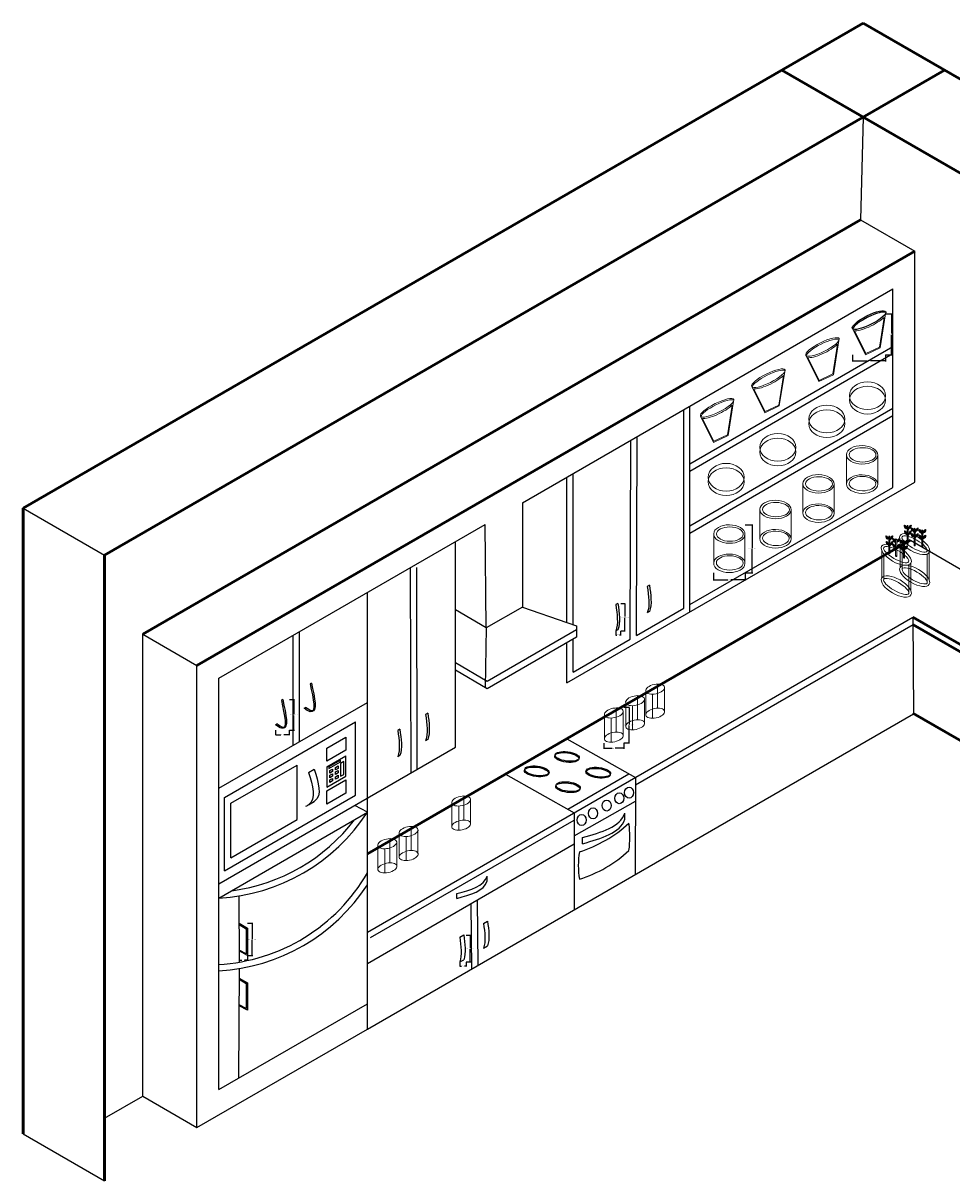
# Model space of a CAD drawing. Units: centimetres. Extents: x 16 to 604, y -284 to 166.
# Tile 1 of 2: x 16 to 312, y -204 to 166. Entities that reach past the tile are written whole.
import ezdxf

# ---------------------------------------------------------------- set-up
doc = ezdxf.new("R2010")
doc.units = ezdxf.units.CM
doc.header["$MEASUREMENT"] = 0
for name, color, linetype, lineweight in [('A-ANNO-DIMS', 2, 'Continuous', 18), ('A-EQPM', 4, 'Continuous', 25), ('A-FLOR-FIXT', 3, 'Continuous', 25), ('A-FURN-ACCS', 9, 'Continuous', 18), ('A-FURN-CASE', 8, 'Continuous', 25), ('A-WALL', 7, 'Continuous', 50)]:
    doc.layers.add(name, color=color, linetype=linetype, lineweight=lineweight)
doc.styles.get("Standard").update_dxf_attribs({"font": 'arial.ttf'})
doc.dimstyles.get("Standard").update_dxf_attribs({"dimtxt": 0.18, "dimasz": 0.18, "dimexe": 0.18, "dimexo": 0.0625, "dimgap": 0.09, "dimtad": 0, "dimtih": 1, "dimtoh": 1, "dimdec": 0, "dimzin": 0, "dimdsep": 46, "dimtxsty": 'Standard', "dimcen": 0.09, "dimadec": 0, "dimazin": 0, "dimtfac": 1, "dimtdec": 0, "dimtofl": 0, "dimtmove": 0, "dimatfit": 3, "dimfxl": 1, "dimtolj": 1, "dimtzin": 0, "dimarcsym": 0})

# ---------------------------------------------------------------- blocks, each defined once
blk = doc.blocks.new('GLASS-TUMBLER')
for p, q in [((0.02, 1.05), (0.02, 8.7)), ((2.21, 0.13), (2.21, 7.72)), ((3.82, 3.25), (3.82, 10.96)), ((6.02, 2.33), (6.02, 9.98))]:
    blk.add_line(p, q)
for centre in [(3.02, 9.34), (3.03, 1.62)]:
    blk.add_ellipse(centre, major_axis=(-3, -0.64), ratio=0.495695)
blk = doc.blocks.new('JAR-STORAGE')
for p, q in [((0, 12.4), (0, 3.03)), ((10, 12.25), (10, 2.89))]:
    blk.add_line(p, q)
for centre, major_axis, ratio in [((5, 12.32), (-5, 0.07), 0.591821), ((5.17, 12.3), (-4.28, 0.05), 0.535916), ((5, 2.96), (-5, 0.07), 0.591821), ((5.13, 3.1), (-4.28, 0.05), 0.535916)]:
    blk.add_ellipse(centre, major_axis=major_axis, ratio=ratio)
blk = doc.blocks.new('CUP')
for p, q in [((8.64, 2.46), (10.15, 11.93)), ((8.83, 2.21), (10.57, 13.1)), ((4.2, 0), (0, 8.4)), ((4.29, 0.38), (0.64, 7.69)), ((4.2, 0), (8.83, 2.21)), ((4.29, 0.38), (8.64, 2.46))]:
    blk.add_line(p, q)
blk.add_ellipse((5.52, 10.63), major_axis=(5.33, 2.67), ratio=0.250569, start_param=3.449003, end_param=5.626799)
blk = doc.blocks.new('HANDLE-FRIDGE')
for p, q in [((0, 10.27), (2.69, 8.71)), ((0, 9.85), (2.26, 8.55)), ((2.26, 8.55), (2.26, 0.52)), ((2.69, 8.71), (2.69, 0)), ((2.69, 8.3), (2.69, 8.3)), ((2.26, 0.52), (0.04, 1.71)), ((2.69, 0), (0.04, 1.42))]:
    blk.add_line(p, q)
blk = doc.blocks.new('MICROWAVE-BUTTON')
for p, q in [((0, 0.81), (0.84, 1.29)), ((0, 0), (0, 0.81)), ((0.84, 0.49), (0, 0)), ((0.84, 1.29), (0.84, 0.49))]:
    blk.add_line(p, q)
blk = doc.blocks.new('HANDLE-CAB-A')
for p, q in [((0.67, 8.79), (0, 8.4)), ((0.67, 0.39), (0, 0))]:
    blk.add_line(p, q)
for points in [[(0, 8.4), (0.44, 5.35), (0.89, 2.29), (0, 0)], [(0.67, 8.79), (1.12, 5.74), (1.56, 2.68), (0.67, 0.39)]]:
    blk.add_open_spline(points, degree=3)
blk = doc.blocks.new('HANDLE-CAB-B')
for p, q in [((2.34, 9.21), (1.89, 8.95)), ((0, 1.14), (0.45, 1.41))]:
    blk.add_line(p, q)
for points in [[(1.89, 8.95), (2.92, 4.2), (4.21, -1.72), (0.69, 0.67), (0, 1.14)], [(2.34, 9.21), (3.37, 4.46), (4.66, -1.46), (1.15, 0.93), (0.45, 1.41)]]:
    blk.add_open_spline(points, degree=3, knots=[0, 0, 0, 0, 8.893101, 11.076836, 11.076836, 11.076836, 11.076836])
blk = doc.blocks.new('HANDLE-CAB-C')
for p, q in [((0, 7.89), (1.27, 8.62)), ((0, 0), (1.27, 0.73))]:
    blk.add_line(p, q)
for points in [[(0, 7.89), (0.38, 5.04), (0.76, 2.19), (0, 0)], [(1.27, 8.62), (1.65, 5.77), (2.03, 2.92), (1.27, 0.73)]]:
    blk.add_open_spline(points, degree=3)
blk = doc.blocks.new('*D13')
at = {"layer": 'A-ANNO-DIMS', "color": 0, "lineweight": -2, "transparency": 16777216}
for p, q in [((246.35, 6.13), (248.77, 6.13)), ((248.59, 5.95), (248.59, -1.37)), ((248.59, -9.05), (248.59, -1.73)), ((246.35, -9.23), (248.77, -9.23))]:
    blk.add_line(p, q, dxfattribs=at)
at = {"layer": 'A-ANNO-DIMS', "color": 0, "transparency": 16777216}
for points in [[(248.56, 5.95), (248.62, 5.95), (248.59, 6.13)], [(248.56, -9.05), (248.62, -9.05), (248.59, -9.23)]]:
    blk.add_solid(points, dxfattribs=at)
at = {"layer": 'Defpoints', "color": 0, "transparency": 16777216}
for p in [(246.29, 6.13), (248.59, 6.13), (246.29, -9.23)]:
    blk.add_point(p, dxfattribs=at)
at = {"layer": 'A-ANNO-DIMS', "color": 0, "transparency": 16777216, "insert": (248.59, -1.55), "char_height": 0.18, "attachment_point": 5}
blk.add_mtext('\\A1;STORAGE JAR 15 TYP.', dxfattribs=at)
blk = doc.blocks.new('*D14')
at = {"layer": 'A-ANNO-DIMS', "color": 0, "lineweight": -2, "transparency": 16777216}
for p, q in [((236.24, -9.3), (236.24, -11.72)), ((246.29, -9.3), (246.29, -11.72)), ((236.42, -11.54), (240.75, -11.54)), ((246.11, -11.54), (241.78, -11.54))]:
    blk.add_line(p, q, dxfattribs=at)
at = {"layer": 'A-ANNO-DIMS', "color": 0, "transparency": 16777216}
for points in [[(236.42, -11.51), (236.42, -11.57), (236.24, -11.54)], [(246.11, -11.51), (246.11, -11.57), (246.29, -11.54)]]:
    blk.add_solid(points, dxfattribs=at)
at = {"layer": 'Defpoints', "color": 0, "transparency": 16777216}
for p in [(236.24, -9.23), (246.29, -9.23), (246.29, -11.54)]:
    blk.add_point(p, dxfattribs=at)
at = {"layer": 'A-ANNO-DIMS', "color": 0, "transparency": 16777216, "insert": (241.27, -11.54), "char_height": 0.18, "attachment_point": 5}
blk.add_mtext('\\A1;10 TYP.', dxfattribs=at)
blk = doc.blocks.new('*D15')
at = {"layer": 'A-ANNO-DIMS', "color": 0, "lineweight": -2, "transparency": 16777216}
for p, q in [((291.2, 73.55), (293.29, 73.55)), ((293.11, 73.37), (293.11, 67.18)), ((293.11, 60.63), (293.11, 66.82)), ((291.2, 60.45), (293.29, 60.45))]:
    blk.add_line(p, q, dxfattribs=at)
at = {"layer": 'A-ANNO-DIMS', "color": 0, "transparency": 16777216}
for points in [[(293.08, 73.37), (293.14, 73.37), (293.11, 73.55)], [(293.08, 60.63), (293.14, 60.63), (293.11, 60.45)]]:
    blk.add_solid(points, dxfattribs=at)
at = {"layer": 'Defpoints', "color": 0, "transparency": 16777216}
for p in [(291.14, 73.55), (293.11, 73.55), (291.14, 60.45)]:
    blk.add_point(p, dxfattribs=at)
at = {"layer": 'A-ANNO-DIMS', "color": 0, "transparency": 16777216, "insert": (293.11, 67), "char_height": 0.18, "attachment_point": 5}
blk.add_mtext('\\A1;CUP 13 TYP.', dxfattribs=at)
blk = doc.blocks.new('*D16')
at = {"layer": 'A-ANNO-DIMS', "color": 0, "lineweight": -2, "transparency": 16777216}
for p, q in [((280.58, 60.39), (280.58, 58.31)), ((291.14, 60.39), (291.14, 58.31)), ((280.76, 58.49), (285.34, 58.49)), ((290.96, 58.49), (286.38, 58.49))]:
    blk.add_line(p, q, dxfattribs=at)
at = {"layer": 'A-ANNO-DIMS', "color": 0, "transparency": 16777216}
for points in [[(280.76, 58.52), (280.76, 58.46), (280.58, 58.49)], [(290.96, 58.52), (290.96, 58.46), (291.14, 58.49)]]:
    blk.add_solid(points, dxfattribs=at)
at = {"layer": 'Defpoints', "color": 0, "transparency": 16777216}
for p in [(280.58, 60.45), (291.14, 60.45), (291.14, 58.49)]:
    blk.add_point(p, dxfattribs=at)
at = {"layer": 'A-ANNO-DIMS', "color": 0, "transparency": 16777216, "insert": (285.86, 58.49), "char_height": 0.18, "attachment_point": 5}
blk.add_mtext('\\A1;11 TYP.', dxfattribs=at)
blk = doc.blocks.new('*D17')
at = {"layer": 'A-ANNO-DIMS', "color": 0, "lineweight": -2, "transparency": 16777216}
for p, q in [((207.57, -52.21), (209.4, -52.21)), ((209.22, -52.39), (209.22, -57.73)), ((209.22, -63.43), (209.22, -58.1)), ((207.57, -63.61), (209.4, -63.61))]:
    blk.add_line(p, q, dxfattribs=at)
at = {"layer": 'A-ANNO-DIMS', "color": 0, "transparency": 16777216}
for points in [[(209.19, -52.39), (209.25, -52.39), (209.22, -52.21)], [(209.19, -63.43), (209.25, -63.43), (209.22, -63.61)]]:
    blk.add_solid(points, dxfattribs=at)
at = {"layer": 'Defpoints', "color": 0, "transparency": 16777216}
for p in [(207.51, -52.21), (209.22, -52.21), (207.51, -63.61)]:
    blk.add_point(p, dxfattribs=at)
at = {"layer": 'A-ANNO-DIMS', "color": 0, "transparency": 16777216, "insert": (209.22, -57.91), "char_height": 0.18, "attachment_point": 5}
blk.add_mtext('\\A1;GLASS TUMBLER 11 TYP.', dxfattribs=at)
blk = doc.blocks.new('*D18')
at = {"layer": 'A-ANNO-DIMS', "color": 0, "lineweight": -2, "transparency": 16777216}
for p, q in [((201.14, -63.68), (201.14, -65.51)), ((201.32, -65.33), (203.86, -65.33)), ((207.33, -65.33), (204.78, -65.33)), ((207.51, -63.68), (207.51, -65.51))]:
    blk.add_line(p, q, dxfattribs=at)
at = {"layer": 'A-ANNO-DIMS', "color": 0, "transparency": 16777216}
for points in [[(201.32, -65.3), (201.32, -65.36), (201.14, -65.33)], [(207.33, -65.3), (207.33, -65.36), (207.51, -65.33)]]:
    blk.add_solid(points, dxfattribs=at)
at = {"layer": 'Defpoints', "color": 0, "transparency": 16777216}
for p in [(201.14, -63.61), (207.51, -63.61), (207.51, -65.33)]:
    blk.add_point(p, dxfattribs=at)
at = {"layer": 'A-ANNO-DIMS', "color": 0, "transparency": 16777216, "insert": (204.32, -65.33), "char_height": 0.18, "attachment_point": 5}
blk.add_mtext('\\A1;6 TYP.', dxfattribs=at)
blk = doc.blocks.new('*D21')
at = {"layer": 'A-ANNO-DIMS', "color": 0, "lineweight": -2, "transparency": 16777216}
for p, q in [((87.31, -121.27), (88.97, -121.27)), ((88.79, -121.45), (88.79, -126.22)), ((88.79, -131.36), (88.79, -126.59)), ((87.31, -131.54), (88.97, -131.54))]:
    blk.add_line(p, q, dxfattribs=at)
at = {"layer": 'A-ANNO-DIMS', "color": 0, "transparency": 16777216}
for points in [[(88.76, -121.45), (88.82, -121.45), (88.79, -121.27)], [(88.76, -131.36), (88.82, -131.36), (88.79, -131.54)]]:
    blk.add_solid(points, dxfattribs=at)
at = {"layer": 'Defpoints', "color": 0, "transparency": 16777216}
for p in [(87.25, -121.27), (88.79, -121.27), (87.25, -131.54)]:
    blk.add_point(p, dxfattribs=at)
at = {"layer": 'A-ANNO-DIMS', "color": 0, "transparency": 16777216, "insert": (88.79, -126.4), "char_height": 0.18, "attachment_point": 5}
blk.add_mtext('\\A1;FRIDGE HANDLE 10 TYP.', dxfattribs=at)
blk = doc.blocks.new('*D22')
at = {"layer": 'A-ANNO-DIMS', "color": 0, "lineweight": -2, "transparency": 16777216}
for p, q in [((84.56, -131.6), (84.56, -133.26)), ((84.74, -133.08), (85.45, -133.08)), ((87.07, -133.08), (86.36, -133.08)), ((87.25, -131.6), (87.25, -133.26))]:
    blk.add_line(p, q, dxfattribs=at)
at = {"layer": 'A-ANNO-DIMS', "color": 0, "transparency": 16777216}
for points in [[(84.74, -133.05), (84.74, -133.11), (84.56, -133.08)], [(87.07, -133.05), (87.07, -133.11), (87.25, -133.08)]]:
    blk.add_solid(points, dxfattribs=at)
at = {"layer": 'Defpoints', "color": 0, "transparency": 16777216}
for p in [(84.56, -131.54), (87.25, -131.54), (87.25, -133.08)]:
    blk.add_point(p, dxfattribs=at)
at = {"layer": 'A-ANNO-DIMS', "color": 0, "transparency": 16777216, "insert": (85.9, -133.08), "char_height": 0.18, "attachment_point": 5}
blk.add_mtext('\\A1;3 TYP.', dxfattribs=at)
blk = doc.blocks.new('*D23')
at = {"layer": 'A-ANNO-DIMS', "color": 0, "lineweight": -2, "transparency": 16777216}
for p, q in [((206.58, -19.03), (208.02, -19.03)), ((207.84, -19.21), (207.84, -23.25)), ((207.84, -27.65), (207.84, -23.61)), ((206.58, -27.83), (208.02, -27.83))]:
    blk.add_line(p, q, dxfattribs=at)
at = {"layer": 'A-ANNO-DIMS', "color": 0, "transparency": 16777216}
for points in [[(207.81, -19.21), (207.87, -19.21), (207.84, -19.03)], [(207.81, -27.65), (207.87, -27.65), (207.84, -27.83)]]:
    blk.add_solid(points, dxfattribs=at)
at = {"layer": 'Defpoints', "color": 0, "transparency": 16777216}
for p in [(206.52, -19.03), (207.84, -19.03), (206.52, -27.83)]:
    blk.add_point(p, dxfattribs=at)
at = {"layer": 'A-ANNO-DIMS', "color": 0, "transparency": 16777216, "insert": (207.84, -23.43), "char_height": 0.18, "attachment_point": 5}
blk.add_mtext('\\A1;CABINET HANDLE A 9 TYP.', dxfattribs=at)
blk = doc.blocks.new('*D24')
at = {"layer": 'A-ANNO-DIMS', "color": 0, "lineweight": -2, "transparency": 16777216}
for p, q in [((204.96, -27.89), (204.96, -29.33)), ((205.14, -29.15), (205.28, -29.15)), ((206.34, -29.15), (206.2, -29.15)), ((206.52, -27.89), (206.52, -29.33))]:
    blk.add_line(p, q, dxfattribs=at)
at = {"layer": 'A-ANNO-DIMS', "color": 0, "transparency": 16777216}
for points in [[(205.14, -29.12), (205.14, -29.18), (204.96, -29.15)], [(206.34, -29.12), (206.34, -29.18), (206.52, -29.15)]]:
    blk.add_solid(points, dxfattribs=at)
at = {"layer": 'Defpoints', "color": 0, "transparency": 16777216}
for p in [(204.96, -27.83), (206.52, -27.83), (206.52, -29.15)]:
    blk.add_point(p, dxfattribs=at)
at = {"layer": 'A-ANNO-DIMS', "color": 0, "transparency": 16777216, "insert": (205.74, -29.15), "char_height": 0.18, "attachment_point": 5}
blk.add_mtext('\\A1;2 TYP.', dxfattribs=at)
blk = doc.blocks.new('*D25')
at = {"layer": 'A-ANNO-DIMS', "color": 0, "lineweight": -2, "transparency": 16777216}
for p, q in [((100.68, -49.77), (102.26, -49.77)), ((102.08, -49.95), (102.08, -54.47)), ((102.08, -59.35), (102.08, -54.84)), ((100.68, -59.53), (102.26, -59.53))]:
    blk.add_line(p, q, dxfattribs=at)
at = {"layer": 'A-ANNO-DIMS', "color": 0, "transparency": 16777216}
for points in [[(102.05, -49.95), (102.11, -49.95), (102.08, -49.77)], [(102.05, -59.35), (102.11, -59.35), (102.08, -59.53)]]:
    blk.add_solid(points, dxfattribs=at)
at = {"layer": 'Defpoints', "color": 0, "transparency": 16777216}
for p in [(100.62, -49.77), (102.08, -49.77), (100.62, -59.53)]:
    blk.add_point(p, dxfattribs=at)
at = {"layer": 'A-ANNO-DIMS', "color": 0, "transparency": 16777216, "insert": (102.08, -54.65), "char_height": 0.18, "attachment_point": 5}
blk.add_mtext('\\A1;CABINET HANDLE B 10 TYP.', dxfattribs=at)
blk = doc.blocks.new('*D26')
at = {"layer": 'A-ANNO-DIMS', "color": 0, "lineweight": -2, "transparency": 16777216}
for p, q in [((96.21, -59.6), (96.21, -61.18)), ((96.39, -61), (97.95, -61)), ((100.44, -61), (98.88, -61)), ((100.62, -59.6), (100.62, -61.18))]:
    blk.add_line(p, q, dxfattribs=at)
at = {"layer": 'A-ANNO-DIMS', "color": 0, "transparency": 16777216}
for points in [[(96.39, -60.97), (96.39, -61.03), (96.21, -61)], [(100.44, -60.97), (100.44, -61.03), (100.62, -61)]]:
    blk.add_solid(points, dxfattribs=at)
at = {"layer": 'Defpoints', "color": 0, "transparency": 16777216}
for p in [(96.21, -59.53), (100.62, -59.53), (100.62, -61)]:
    blk.add_point(p, dxfattribs=at)
at = {"layer": 'A-ANNO-DIMS', "color": 0, "transparency": 16777216, "insert": (98.42, -61), "char_height": 0.18, "attachment_point": 5}
blk.add_mtext('\\A1;4 TYP.', dxfattribs=at)
blk = doc.blocks.new('*D27')
at = {"layer": 'A-ANNO-DIMS', "color": 0, "lineweight": -2, "transparency": 16777216}
for p, q in [((157.2, -125.02), (158.61, -125.02)), ((158.43, -125.2), (158.43, -129.14)), ((158.43, -133.45), (158.43, -129.51)), ((157.2, -133.63), (158.61, -133.63))]:
    blk.add_line(p, q, dxfattribs=at)
at = {"layer": 'A-ANNO-DIMS', "color": 0, "transparency": 16777216}
for points in [[(158.4, -125.2), (158.46, -125.2), (158.43, -125.02)], [(158.4, -133.45), (158.46, -133.45), (158.43, -133.63)]]:
    blk.add_solid(points, dxfattribs=at)
at = {"layer": 'Defpoints', "color": 0, "transparency": 16777216}
for p in [(157.14, -125.02), (158.43, -125.02), (157.14, -133.63)]:
    blk.add_point(p, dxfattribs=at)
at = {"layer": 'A-ANNO-DIMS', "color": 0, "transparency": 16777216, "insert": (158.43, -129.32), "char_height": 0.18, "attachment_point": 5}
blk.add_mtext('\\A1;CABINET HANDLE C 9 TYP.', dxfattribs=at)
blk = doc.blocks.new('*D28')
at = {"layer": 'A-ANNO-DIMS', "color": 0, "lineweight": -2, "transparency": 16777216}
for p, q in [((155.11, -133.7), (155.11, -135.11)), ((155.29, -134.93), (155.67, -134.93)), ((156.96, -134.93), (156.58, -134.93)), ((157.14, -133.7), (157.14, -135.11))]:
    blk.add_line(p, q, dxfattribs=at)
at = {"layer": 'A-ANNO-DIMS', "color": 0, "transparency": 16777216}
for points in [[(155.29, -134.9), (155.29, -134.96), (155.11, -134.93)], [(156.96, -134.9), (156.96, -134.96), (157.14, -134.93)]]:
    blk.add_solid(points, dxfattribs=at)
at = {"layer": 'Defpoints', "color": 0, "transparency": 16777216}
for p in [(155.11, -133.63), (157.14, -133.63), (157.14, -134.93)]:
    blk.add_point(p, dxfattribs=at)
at = {"layer": 'A-ANNO-DIMS', "color": 0, "transparency": 16777216, "insert": (156.13, -134.93), "char_height": 0.18, "attachment_point": 5}
blk.add_mtext('\\A1;2 TYP.', dxfattribs=at)

msp = doc.modelspace()

# ---------------------------------------------------------------- linework, layer by layer
at = {"layer": 'A-EQPM'}
for p, q in [((191.32, -25.81), (191.32, 22.45)), ((189.32, -25.11), (189.32, 21.3)), ((175.17, 13.13), (175.17, -20.2)), ((163.6, -26.88), (163.19, 6.21)), ((175.17, -20.2), (163.6, -26.88)), ((175.17, -20.2), (189.32, -25.11)), ((125.6, -124.13), (299.95, -23.47)), ((189.32, -25.11), (192.42, -26.18)), ((163.6, -26.88), (163.26, -46)), ((192.42, -27.53), (163.85, -44.02)), ((192.42, -26.18), (192.42, -29.84)), ((192.42, -29.84), (163.83, -46.34)), ((189.32, -44.45), (189.32, -31.63)), ((191.32, -40.98), (209.6, -30.43)), ((191.32, -40.98), (191.32, -30.47)), ((78.11, -78.11), (125.6, -50.69)), ((125.6, -155.06), (300.07, -54.33)), ((79.89, -81.04), (121.75, -56.88)), ((121.75, -80.29), (121.75, -56.88)), ((112.59, -65.26), (118.65, -61.76)), ((118.65, -61.76), (118.65, -65.96)), ((189.32, -62.28), (211.28, -74.66)), ((78.11, -108.66), (153.72, -65)), ((112.59, -69.46), (112.59, -65.26)), ((118.65, -65.96), (112.59, -69.46)), ((112.59, -71.25), (118.65, -67.75)), ((117.02, -69.09), (113.32, -71.22)), ((113.32, -71.76), (117.02, -69.62)), ((118.1, -69.55), (117.01, -70.18)), ((117.01, -70.18), (117.01, -74.3)), ((117.02, -69.62), (117.02, -69.09)), ((118.1, -73.67), (118.1, -69.55)), ((118.65, -74.28), (118.65, -67.75)), ((81.99, -82.92), (103.1, -70.74)), ((103.1, -88.12), (103.1, -70.74)), ((106.77, -73.07), (108.6, -72.02)), ((112.59, -71.25), (112.59, -77.78)), ((113.32, -71.22), (113.32, -71.76)), ((117.01, -74.3), (118.1, -73.67)), ((169.76, -73.57), (191.72, -85.95)), ((189.63, -84.78), (209.16, -73.46)), ((112.59, -77.78), (118.65, -74.28)), ((112.59, -78.94), (118.65, -75.45)), ((118.65, -75.45), (118.65, -79.65)), ((211.28, -74.66), (211.21, -105.64)), ((79.89, -104.46), (121.75, -80.29)), ((112.59, -83.15), (112.59, -78.94)), ((118.65, -79.65), (112.59, -83.15)), ((125.6, -155.06), (125.6, -81.24)), ((106.77, -83.41), (108.6, -82.35)), ((125.6, -85.78), (121.53, -83.58)), ((191.7, -93.27), (211.27, -82.24)), ((78.11, -113.24), (125.6, -85.78)), ((81.99, -100.3), (103.1, -88.12)), ((191.72, -85.95), (191.65, -116.93)), ((207.89, -88.03), (207.89, -86.07)), ((194.38, -95.83), (194.38, -93.87)), ((78.11, -174.4), (125.6, -146.98))]:
    msp.add_line(p, q, dxfattribs=at)
for centre, radius, start, end in [((74.69, -52.54), 60.8, 273.2228, 326.864), ((74.69, -52.54), 58.8, 277.3793, 322.7074), ((180.06, -57.12), 43.41, 287.8539, 312.1461), ((175.12, -93.67), 34.34, 352.7074, 7.2926), ((218.44, -102.8), 25.45, 170.1385, 189.8615), ((181.2, -67.82), 41.18, 287.1858, 312.8142), ((74.69, -75.74), 58.8, 273.2228, 329.981), ((74.69, -75.74), 60.8, 273.2228, 326.864)]:
    msp.add_arc(centre, radius, start, end, dxfattribs=at)
for centre, major_axis, ratio in [((189.34, -68.27), (-3.87, 0.48), 0.385589), ((189.44, -67.93), (-3.87, 0.48), 0.385589), ((179.66, -72.89), (-3.87, 0.48), 0.385589), ((179.76, -72.55), (-3.87, 0.48), 0.385589), ((199.31, -73.32), (-3.87, 0.48), 0.385589), ((199.42, -72.98), (-3.87, 0.48), 0.385589), ((189.64, -77.94), (-3.87, 0.48), 0.385589), ((189.74, -77.6), (-3.87, 0.48), 0.385589), ((206.1, -81.3), (0, 1.76), 0.821496), ((209.23, -79.5), (0, 1.76), 0.821496), ((197.71, -86.15), (0, 1.76), 0.821496), ((202.07, -83.63), (0, 1.76), 0.821496), ((194.06, -88.26), (0, 1.76), 0.821496)]:
    msp.add_ellipse(centre, major_axis=major_axis, ratio=ratio, dxfattribs=at)
for points in [[(106.77, -73.07), (108.12, -77.3), (109.61, -81.96), (106.17, -83.77), (105.85, -83.93)], [(108.6, -72.02), (109.95, -76.24), (111.44, -80.9), (108, -82.71), (107.68, -82.88)]]:
    msp.add_open_spline(points, degree=3, knots=[0, 0, 0, 0, 10.334335, 11.39113, 11.39113, 11.39113, 11.39113], dxfattribs=at)
for points in [[(194.38, -93.87), (200.41, -92.15), (206.44, -90.43), (207.89, -86.07)], [(194.38, -95.83), (200.41, -94.11), (206.44, -92.39), (207.89, -88.03)]]:
    msp.add_open_spline(points, degree=3, dxfattribs=at)
at = {"layer": 'A-FLOR-FIXT'}
msp.add_line((299.16, 1.14), (469.25, -97.06), dxfattribs=at)
at = {"layer": 'A-FURN-ACCS'}
for p, q in [((297.78, 4.92), (297.2, 5.94)), ((297.78, 4.9), (297.2, 5.92)), ((297.86, 3.11), (297.28, 4.14)), ((297.86, 3.1), (297.28, 4.12)), ((298.11, 0.43), (298.11, 5.83)), ((298.44, 4.54), (298.69, 4.9)), ((298.45, 0.26), (298.45, 5.65)), ((298.45, 4.53), (298.69, 4.89)), ((298.72, 4.96), (299.38, 5.93)), ((298.72, 3.14), (299.38, 4.12)), ((298.73, 4.94), (299.38, 5.92)), ((298.73, 3.12), (299.38, 4.1)), ((300.03, 4.02), (299.45, 5.05)), ((300.04, 4.04), (299.46, 5.06)), ((300.28, 3.6), (300.07, 3.98)), ((300.28, 3.58), (300.07, 3.97)), ((300.28, -0.46), (300.28, 4.94)), ((300.61, 3.65), (300.86, 4.01)), ((300.62, -0.63), (300.62, 4.76)), ((300.62, 3.63), (300.86, 3.99)), ((300.89, 4.06), (301.55, 5.04)), ((300.89, 4.05), (301.55, 5.02)), ((302.49, 3.51), (301.91, 4.54)), ((302.5, 3.53), (301.92, 4.56)), ((302.74, -0.97), (302.74, 4.43)), ((303.08, -1.14), (303.08, 4.25)), ((303.35, 3.56), (304.01, 4.53)), ((303.35, 3.54), (304.01, 4.51)), ((291.91, 1.51), (291.32, 2.53)), ((291.91, 1.52), (291.33, 2.55)), ((291.99, -0.3), (291.4, 0.73)), ((291.99, -0.28), (291.41, 0.75)), ((292.24, -2.96), (292.24, 2.44)), ((292.57, -3.13), (292.57, 2.26)), ((292.57, 1.15), (292.81, 1.51)), ((292.57, 1.14), (292.82, 1.5)), ((292.85, 1.57), (293.51, 2.54)), ((292.85, 1.55), (293.51, 2.52)), ((292.85, -0.25), (293.51, 0.73)), ((292.85, -0.27), (293.51, 0.71)), ((294.16, 0.65), (293.58, 1.67)), ((294.16, 0.63), (293.58, 1.65)), ((294.41, 0.21), (294.19, 0.59)), ((294.41, 0.19), (294.19, 0.58)), ((294.41, -3.85), (294.41, 1.54)), ((294.74, -4.02), (294.74, 1.37)), ((294.74, 0.26), (294.98, 0.61)), ((294.74, 0.24), (294.98, 0.6)), ((295.02, 0.67), (295.68, 1.65)), ((295.02, 0.65), (295.68, 1.63)), ((295.81, -7.53), (295.81, 1.32)), ((296.62, 0.14), (296.04, 1.16)), ((296.62, 0.12), (296.04, 1.15)), ((296.51, -7.93), (296.51, 0.16)), ((296.87, -0.32), (296.65, 0.07)), ((296.87, -0.29), (296.66, 0.09)), ((296.87, -4.36), (296.87, 1.04)), ((297.2, -4.53), (297.2, 0.86)), ((297.2, -0.25), (297.44, 0.11)), ((297.2, -0.27), (297.44, 0.09)), ((297.48, 0.16), (298.14, 1.14)), ((297.48, 0.15), (298.14, 1.12)), ((297.89, 3.05), (298.11, 2.74)), ((297.89, 3.04), (298.11, 2.73)), ((298.42, -0.09), (298.21, 0.3)), ((298.44, 2.73), (298.69, 3.09)), ((298.45, 2.71), (298.69, 3.07)), ((300.03, 2.26), (299.45, 3.28)), ((300.04, 2.28), (299.46, 3.3)), ((300.28, 1.84), (300.07, 2.22)), ((300.28, 1.82), (300.07, 2.2)), ((300.61, 1.83), (300.86, 2.19)), ((300.62, 1.82), (300.86, 2.18)), ((300.89, 2.25), (301.55, 3.23)), ((300.89, 2.23), (301.55, 3.21)), ((302.49, 1.75), (301.91, 2.77)), ((302.5, 1.77), (301.92, 2.79)), ((302.74, 3.11), (302.53, 3.48)), ((302.74, 3.08), (302.53, 3.46)), ((302.74, 1.31), (302.53, 1.69)), ((303.07, 3.14), (303.32, 3.5)), ((303.07, 1.32), (303.32, 1.68)), ((303.08, 3.13), (303.32, 3.49)), ((303.08, 1.31), (303.32, 1.67)), ((303.35, 1.74), (304.01, 2.72)), ((303.35, 1.72), (304.01, 2.7)), ((289.94, -10.92), (289.94, -2.07)), ((290.63, -11.32), (290.63, -3.23)), ((292.02, -0.34), (292.24, -0.65)), ((292.02, -0.35), (292.24, -0.67)), ((292.57, -0.67), (292.81, -0.31)), ((292.57, -0.68), (292.82, -0.32)), ((294.16, -1.12), (293.58, -0.09)), ((294.16, -1.13), (293.58, -0.11)), ((295.02, -1.14), (295.68, -0.17)), ((295.02, -1.16), (295.68, -0.18)), ((296.62, -1.62), (296.04, -0.6)), ((296.62, -1.64), (296.04, -0.62)), ((296.87, -2.08), (296.65, -1.7)), ((297.2, -2.07), (297.44, -1.71)), ((297.2, -2.08), (297.44, -1.72)), ((297.48, -1.65), (298.14, -0.67)), ((297.48, -1.67), (298.14, -0.69)), ((304.53, -12.13), (304.53, -3.28)), ((305.17, -11.61), (305.17, -2.76)), ((298.66, -15.52), (298.66, -6.68)), ((299.29, -15), (299.29, -6.15))]:
    msp.add_line(p, q, dxfattribs=at)
for centre, radius, start, end in [((298.08, 5.75), 0.948, 165.5656, 253.6185), ((296.94, 5.11), 0.911, 343.2915, 75.8926), ((296.94, 5.11), 0.911, 343.2915, 75.8926), ((298.13, 5.77), 0.948, 169.4469, 248.0113), ((296.89, 5.09), 0.911, 347.5333, 69.9249), ((296.89, 5.09), 0.911, 347.5333, 69.9249), ((298.16, 3.95), 0.948, 165.5656, 253.6185), ((297.02, 3.3), 0.911, 343.2915, 75.8926), ((297.02, 3.3), 0.911, 343.2915, 75.8926), ((298.21, 3.97), 0.948, 169.4469, 248.0113), ((296.97, 3.28), 0.911, 347.5333, 69.9249), ((296.97, 3.28), 0.911, 347.5333, 69.9249), ((299.58, 5.08), 0.911, 99.666, 192.2671), ((299.58, 5.08), 0.911, 99.666, 192.2671), ((299.58, 3.27), 0.911, 99.666, 192.2671), ((299.58, 3.27), 0.911, 99.666, 192.2671), ((298.49, 5.81), 0.948, 281.9401, 9.993), ((298.49, 4), 0.948, 281.9401, 9.993), ((299.63, 5.06), 0.911, 105.6338, 188.0253), ((299.63, 5.06), 0.911, 105.6338, 188.0253), ((299.63, 3.24), 0.911, 105.6338, 188.0253), ((299.63, 3.24), 0.911, 105.6338, 188.0253), ((298.44, 5.83), 0.948, 287.5473, 6.1118), ((298.44, 4.02), 0.948, 287.5473, 6.1118), ((300.33, 4.88), 0.948, 165.5656, 253.6185), ((299.19, 4.23), 0.911, 343.2915, 75.8926), ((299.19, 4.23), 0.911, 343.2915, 75.8926), ((300.39, 4.89), 0.948, 169.4469, 248.0113), ((299.14, 4.21), 0.911, 347.5333, 69.9249), ((299.14, 4.21), 0.911, 347.5333, 69.9249), ((301.75, 4.19), 0.911, 99.666, 192.2671), ((301.75, 4.19), 0.911, 99.666, 192.2671), ((300.66, 4.92), 0.948, 281.9401, 9.993), ((301.8, 4.16), 0.911, 105.6338, 188.0253), ((301.8, 4.16), 0.911, 105.6338, 188.0253), ((300.61, 4.94), 0.948, 287.5473, 6.1118), ((302.79, 4.37), 0.948, 165.5656, 253.6185), ((301.65, 3.72), 0.911, 343.2915, 75.8926), ((301.65, 3.72), 0.911, 343.2915, 75.8926), ((302.85, 4.38), 0.948, 169.4469, 248.0113), ((301.6, 3.7), 0.911, 347.5333, 69.9249), ((301.6, 3.7), 0.911, 347.5333, 69.9249), ((304.21, 3.68), 0.911, 99.666, 192.2671), ((304.21, 3.68), 0.911, 99.666, 192.2671), ((303.12, 4.41), 0.948, 281.9401, 9.993), ((304.26, 3.66), 0.911, 105.6338, 188.0253), ((304.26, 3.66), 0.911, 105.6338, 188.0253), ((303.07, 4.43), 0.948, 287.5473, 6.1118), ((292.2, 2.36), 0.948, 165.5656, 253.6185), ((291.06, 1.71), 0.911, 343.2915, 75.8926), ((291.06, 1.71), 0.911, 343.2915, 75.8926), ((292.26, 2.38), 0.948, 169.4469, 248.0113), ((291.01, 1.69), 0.911, 347.5333, 69.9249), ((291.01, 1.69), 0.911, 347.5333, 69.9249), ((292.28, 0.56), 0.948, 165.5656, 253.6185), ((291.14, -0.09), 0.911, 343.2915, 75.8926), ((291.14, -0.09), 0.911, 343.2915, 75.8926), ((292.34, 0.57), 0.948, 169.4469, 248.0113), ((291.09, -0.11), 0.911, 347.5333, 69.9249), ((291.09, -0.11), 0.911, 347.5333, 69.9249), ((293.71, 1.69), 0.911, 99.666, 192.2671), ((293.71, 1.69), 0.911, 99.666, 192.2671), ((293.71, -0.13), 0.911, 99.666, 192.2671), ((293.71, -0.13), 0.911, 99.666, 192.2671), ((292.62, 2.42), 0.948, 281.9401, 9.993), ((292.62, 0.61), 0.948, 281.9401, 9.993), ((293.75, 1.66), 0.911, 105.6338, 188.0253), ((293.75, 1.66), 0.911, 105.6338, 188.0253), ((293.75, -0.15), 0.911, 105.6338, 188.0253), ((293.75, -0.15), 0.911, 105.6338, 188.0253), ((292.57, 2.44), 0.948, 287.5473, 6.1118), ((292.57, 0.63), 0.948, 287.5473, 6.1118), ((294.46, 1.48), 0.948, 165.5656, 253.6185), ((293.32, 0.84), 0.911, 343.2915, 75.8926), ((293.32, 0.84), 0.911, 343.2915, 75.8926), ((294.51, 1.5), 0.948, 169.4469, 248.0113), ((293.27, 0.82), 0.911, 347.5333, 69.9249), ((293.27, 0.82), 0.911, 347.5333, 69.9249), ((295.87, 0.8), 0.911, 99.666, 192.2671), ((295.87, 0.8), 0.911, 99.666, 192.2671), ((294.79, 1.53), 0.948, 281.9401, 9.993), ((295.92, 0.77), 0.911, 105.6338, 188.0253), ((295.92, 0.77), 0.911, 105.6338, 188.0253), ((294.73, 1.55), 0.948, 287.5473, 6.1118), ((296.92, 0.98), 0.948, 165.5656, 253.6185), ((295.78, 0.33), 0.911, 343.2915, 75.8926), ((295.78, 0.33), 0.911, 343.2915, 75.8926), ((296.97, 0.99), 0.948, 169.4469, 248.0113), ((295.73, 0.31), 0.911, 347.5333, 69.9249), ((295.73, 0.31), 0.911, 347.5333, 69.9249), ((298.34, 0.29), 0.911, 99.666, 192.2671), ((298.34, 0.29), 0.911, 99.666, 192.2671), ((297.25, 1.02), 0.948, 281.9401, 9.993), ((298.38, 0.26), 0.911, 105.6338, 188.0253), ((298.38, 0.26), 0.911, 105.6338, 188.0253), ((297.2, 1.04), 0.948, 287.5473, 6.1118), ((300.33, 3.11), 0.948, 165.5656, 253.6185), ((299.19, 2.47), 0.911, 343.2915, 75.8926), ((299.19, 2.47), 0.911, 343.2915, 75.8926), ((300.39, 3.13), 0.948, 169.4469, 248.0113), ((299.14, 2.44), 0.911, 347.5333, 69.9249), ((299.14, 2.44), 0.911, 347.5333, 69.9249), ((301.75, 2.37), 0.911, 99.666, 192.2671), ((301.75, 2.37), 0.911, 99.666, 192.2671), ((300.66, 3.11), 0.948, 281.9401, 9.993), ((301.8, 2.35), 0.911, 105.6338, 188.0253), ((301.8, 2.35), 0.911, 105.6338, 188.0253), ((300.61, 3.13), 0.948, 287.5473, 6.1118), ((302.79, 2.6), 0.948, 165.5656, 253.6185), ((301.65, 1.96), 0.911, 343.2915, 75.8926), ((301.65, 1.96), 0.911, 343.2915, 75.8926), ((302.85, 2.62), 0.948, 169.4469, 248.0113), ((301.6, 1.94), 0.911, 347.5333, 69.9249), ((301.6, 1.94), 0.911, 347.5333, 69.9249), ((304.21, 1.87), 0.911, 99.666, 192.2671), ((304.21, 1.87), 0.911, 99.666, 192.2671), ((303.12, 2.6), 0.948, 281.9401, 9.993), ((304.26, 1.84), 0.911, 105.6338, 188.0253), ((304.26, 1.84), 0.911, 105.6338, 188.0253), ((303.07, 2.62), 0.948, 287.5473, 6.1118), ((294.46, -0.28), 0.948, 165.5656, 253.6185), ((293.32, -0.93), 0.911, 343.2915, 75.8926), ((293.32, -0.93), 0.911, 343.2915, 75.8926), ((294.51, -0.26), 0.948, 169.4469, 248.0113), ((293.27, -0.95), 0.911, 347.5333, 69.9249), ((293.27, -0.95), 0.911, 347.5333, 69.9249), ((295.87, -1.02), 0.911, 99.666, 192.2671), ((295.87, -1.02), 0.911, 99.666, 192.2671), ((294.79, -0.28), 0.948, 281.9401, 9.993), ((295.92, -1.04), 0.911, 105.6338, 188.0253), ((295.92, -1.04), 0.911, 105.6338, 188.0253), ((294.73, -0.27), 0.948, 287.5473, 6.1118), ((296.92, -0.79), 0.948, 165.5656, 253.6185), ((295.78, -1.44), 0.911, 343.2915, 75.8926), ((295.78, -1.44), 0.911, 343.2915, 75.8926), ((296.97, -0.77), 0.948, 169.4469, 248.0113), ((295.73, -1.46), 0.911, 347.5333, 69.9249), ((295.73, -1.46), 0.911, 347.5333, 69.9249), ((298.34, -1.53), 0.911, 99.666, 192.2671), ((298.34, -1.53), 0.911, 99.666, 192.2671), ((297.25, -0.79), 0.948, 281.9401, 9.993), ((298.38, -1.55), 0.911, 105.6338, 188.0253), ((298.38, -1.55), 0.911, 105.6338, 188.0253), ((297.2, -0.77), 0.948, 287.5473, 6.1118)]:
    msp.add_arc(centre, radius, start, end, dxfattribs=at)
for centre, major_axis, ratio in [((271.01, 62.91), (5.33, 2.67), 0.250569), ((253.73, 52.94), (5.33, 2.67), 0.250569), ((285.41, 47.37), (-5.75, 0), 0.770727), ((285.41, 45.93), (-5.75, 0), 0.770727), ((237.36, 43.48), (5.33, 2.67), 0.250569), ((272.43, 39.88), (-5.75, 0), 0.770727), ((272.43, 38.43), (-5.75, 0), 0.770727), ((256.74, 30.82), (-5.75, 0), 0.770727), ((256.74, 29.37), (-5.75, 0), 0.770727), ((240.24, 21.29), (-5.75, 0), 0.770727), ((240.24, 19.85), (-5.75, 0), 0.770727), ((300.49, -0.06), (-4.68, 2.7), 0.441812), ((298.28, 5.75), (-0.167, 0.096), 0.263512), ((300.45, 4.86), (-0.167, 0.096), 0.263512), ((302.91, 4.35), (-0.167, 0.096), 0.263512), ((294.61, -3.45), (-4.68, 2.7), 0.441812), ((292.41, 2.36), (-0.167, 0.096), 0.263512), ((294.57, 1.47), (-0.167, 0.096), 0.263512), ((300.46, -0.04), (-3.98, 2.3), 0.306783), ((297.04, 0.96), (-0.167, 0.096), 0.263512), ((298.28, 0.34), (-0.167, 0.096), 0.311769), ((294.58, -3.44), (-3.98, 2.3), 0.306783), ((292.41, -3.06), (-0.167, 0.096), 0.311769), ((300.45, -0.56), (-0.167, 0.096), 0.311769), ((302.91, -1.06), (-0.167, 0.096), 0.311769), ((294.57, -3.95), (-0.167, 0.096), 0.311769), ((300.49, -10.23), (-4.68, 2.7), 0.441812), ((300.49, -10.23), (-3.98, 2.3), 0.306783), ((297.04, -4.46), (-0.167, 0.096), 0.311769), ((294.61, -13.62), (-4.68, 2.7), 0.441812), ((294.61, -13.62), (-3.98, 2.3), 0.306783)]:
    msp.add_ellipse(centre, major_axis=major_axis, ratio=ratio, dxfattribs=at)
for centre in [(271.2, 62.48), (253.92, 52.51), (237.55, 43.06)]:
    msp.add_ellipse(centre, major_axis=(5.33, 2.67), ratio=0.250569, start_param=0.144822, end_param=2.971969, dxfattribs=at)
at = {"layer": 'A-FURN-CASE'}
for p, q in [((284.05, 136.41), (283.21, 103.59)), ((283.21, 103.59), (300.53, 93.59)), ((300.53, 19.76), (300.53, 93.59)), ((175.17, 13.13), (293.53, 81.47)), ((293.53, 18.03), (293.53, 81.47)), ((293.53, 62.99), (228.67, 25.42)), ((293.53, 60.68), (228.67, 23.11)), ((248.08, 49.63), (248.08, 49.64)), ((226.67, -20.58), (226.67, 42.86)), ((228.67, -21.73), (228.67, 44.02)), ((293.53, 43.22), (228.67, 5.64)), ((293.53, 40.9), (228.67, 3.33)), ((211.61, -29.27), (211.77, 34.26)), ((209.6, -30.43), (209.77, 33.1)), ((189.32, -44.45), (300.53, 19.76)), ((228.67, -19.42), (293.53, 18.03)), ((15.58, 11.41), (41.56, -3.59)), ((78.11, -42.91), (163.19, 6.21)), ((153.72, -65), (153.72, 0.74)), ((139.53, -73.2), (139.4, -7.52)), ((141.52, -72.04), (141.4, -7.52)), ((125.6, -81.24), (125.6, -15.49)), ((163.6, -26.88), (153.72, -21.08)), ((211.61, -29.27), (226.67, -20.58)), ((211.28, -76.97), (299.96, -25.77)), ((299.95, -23.47), (300.07, -54.33)), ((53.79, -28.87), (71.11, -38.87)), ((53.79, -176.53), (53.79, -28.87)), ((101.85, -64.4), (101.88, -29.19)), ((103.86, -63.25), (103.88, -28.03)), ((71.11, -186.53), (71.11, -38.87)), ((163.85, -44.02), (153.72, -37.99)), ((163.83, -46.34), (153.72, -40.32)), ((78.11, -174.4), (78.11, -42.91)), ((79.89, -104.46), (79.89, -81.04)), ((81.99, -100.3), (81.99, -82.92)), ((126.6, -125.86), (191.71, -88.26)), ((125.6, -134.15), (191.7, -95.86)), ((163.86, -107.74), (163.86, -106.22)), ((84.52, -112.54), (84.61, -133.69)), ((154.2, -113.32), (154.2, -111.8)), ((160.63, -113.86), (160.89, -134.69)), ((158.65, -115.01), (158.9, -135.84)), ((84.62, -135.72), (84.45, -170.74)), ((71.11, -186.53), (125.6, -155.06)), ((41.56, -183.59), (53.79, -176.53)), ((53.79, -176.53), (71.11, -186.53)), ((15.58, -188.59), (41.56, -203.59))]:
    msp.add_line(p, q, dxfattribs=at)
msp.add_arc((74.69, -52.54), 58.8, 273.2228, 273.3325, dxfattribs=at)
msp.add_ellipse((285.91, 71.51), major_axis=(5.33, 2.67), ratio=0.250569, dxfattribs=at)
msp.add_ellipse((286.1, 71.08), major_axis=(5.33, 2.67), ratio=0.250569, start_param=0.144822, end_param=2.971969, dxfattribs=at)
for points in [[(154.2, -111.8), (158.56, -110.6), (162.92, -109.4), (163.86, -106.22)], [(154.2, -113.32), (158.56, -112.12), (162.92, -110.92), (163.86, -107.74)]]:
    msp.add_open_spline(points, degree=3, dxfattribs=at)
at = {"layer": 'A-WALL'}
for p, q in [((15.58, 11.41), (284.05, 166.41)), ((284.05, 166.41), (604.48, -18.59)), ((41.56, -3.59), (310.03, 151.41)), ((578.5, -33.59), (258.07, 151.41)), ((53.79, -28.87), (283.21, 103.59)), ((71.11, -38.87), (300.53, 93.59)), ((15.58, 11.41), (15.58, -188.59)), ((125.6, -99.06), (299.16, 1.14)), ((41.56, -203.59), (41.56, -3.59)), ((299.95, -23.47), (469.25, -121.22)), ((299.95, -23.47), (469.25, -121.22)), ((299.95, -25.78), (469.25, -123.52)), ((299.95, -54.11), (470.03, -152.31))]:
    msp.add_line(p, q, dxfattribs=at)

# ---------------------------------------------------------------- block references
at = {"layer": 'A-EQPM'}
for name, p in [('MICROWAVE-BUTTON', (113.62, -73.29)), ('MICROWAVE-BUTTON', (113.62, -74.75)), ('MICROWAVE-BUTTON', (115.43, -72.24)), ('MICROWAVE-BUTTON', (115.43, -73.71)), ('MICROWAVE-BUTTON', (115.43, -75.22)), ('MICROWAVE-BUTTON', (113.62, -76.26)), ('HANDLE-FRIDGE', (84.56, -131.54)), ('HANDLE-FRIDGE', (84.57, -149.03))]:
    msp.add_blockref(name, p, dxfattribs=at)
at = {"layer": 'A-FURN-ACCS'}
for name, p in [('CUP', (280.58, 60.45)), ('CUP', (265.68, 51.85)), ('CUP', (248.4, 41.87)), ('CUP', (232.03, 32.42)), ('JAR-STORAGE', (278.67, 16.14)), ('JAR-STORAGE', (264.74, 6.86)), ('JAR-STORAGE', (251, -1.34)), ('JAR-STORAGE', (236.26, -9.19)), ('GLASS-TUMBLER', (214.53, -55.76)), ('GLASS-TUMBLER', (208.11, -59.46)), ('GLASS-TUMBLER', (201.3, -63.39)), ('GLASS-TUMBLER', (152.56, -91.53)), ('GLASS-TUMBLER', (135.74, -101.25)), ('GLASS-TUMBLER', (128.94, -105.17))]:
    msp.add_blockref(name, p, dxfattribs=at)
at = {"layer": 'A-FURN-CASE'}
for name, p in [('HANDLE-CAB-A', (215.05, -22)), ('HANDLE-CAB-A', (204.96, -27.83)), ('HANDLE-CAB-B', (105.38, -53.69)), ('HANDLE-CAB-B', (96.21, -58.98)), ('HANDLE-CAB-A', (144.19, -62.91)), ('HANDLE-CAB-A', (135.28, -68.05)), ('HANDLE-CAB-C', (162.71, -129.25)), ('HANDLE-CAB-C', (155.11, -133.63))]:
    msp.add_blockref(name, p, dxfattribs=at)

# ---------------------------------------------------------------- dimensions: what is measured, and where the dimension line sits
at = {"layer": 'A-ANNO-DIMS'}
for base, p1, p2, text, picture, middle in [((293.11, 73.55), (291.14, 60.45), (291.14, 73.55), 'CUP <> TYP.', '*D15', (293.11, 67)), ((248.59, 6.13), (246.29, -9.23), (246.29, 6.13), 'STORAGE JAR <> TYP.', '*D13', (248.59, -1.55)), ((207.84, -19.03), (206.52, -27.83), (206.52, -19.03), 'CABINET HANDLE A <> TYP.', '*D23', (207.84, -23.43)), ((102.08, -49.77), (100.62, -59.53), (100.62, -49.77), 'CABINET HANDLE B <> TYP.', '*D25', (102.08, -54.65)), ((209.22, -52.21), (207.51, -63.61), (207.51, -52.21), 'GLASS TUMBLER <> TYP.', '*D17', (209.22, -57.91)), ((88.79, -121.27), (87.25, -131.54), (87.25, -121.27), 'FRIDGE HANDLE <> TYP.', '*D21', (88.79, -126.4)), ((158.43, -125.02), (157.14, -133.63), (157.14, -125.02), 'CABINET HANDLE C <> TYP.', '*D27', (158.43, -129.32))]:
    dim = msp.add_linear_dim(base=base, p1=p1, p2=p2, angle=90, text=text, dimstyle='Standard', override={"dimdec": 0, "dimlfac": 1, "dimrnd": 0, "dimzin": 0, "dimdsep": 46, "dimlunit": 2}, dxfattribs=at)
    dim.commit()
    dim.dimension.update_dxf_attribs({"geometry": picture, "text_midpoint": middle})
for base, p1, p2, picture, middle in [((291.14, 58.49), (280.58, 60.45), (291.14, 60.45), '*D16', (285.86, 58.49)), ((246.29, -11.54), (236.24, -9.23), (246.29, -9.23), '*D14', (241.27, -11.54)), ((206.52, -29.15), (204.96, -27.83), (206.52, -27.83), '*D24', (205.74, -29.15)), ((100.62, -61), (96.21, -59.53), (100.62, -59.53), '*D26', (98.42, -61)), ((207.51, -65.33), (201.14, -63.61), (207.51, -63.61), '*D18', (204.32, -65.33)), ((87.25, -133.08), (84.56, -131.54), (87.25, -131.54), '*D22', (85.9, -133.08)), ((157.14, -134.93), (155.11, -133.63), (157.14, -133.63), '*D28', (156.13, -134.93))]:
    dim = msp.add_linear_dim(base=base, p1=p1, p2=p2, text='<> TYP.', dimstyle='Standard', override={"dimdec": 0, "dimlfac": 1, "dimrnd": 0, "dimzin": 0, "dimdsep": 46, "dimlunit": 2}, dxfattribs=at)
    dim.commit()
    dim.dimension.update_dxf_attribs({"geometry": picture, "text_midpoint": middle})

doc.saveas('drawing.dxf')
